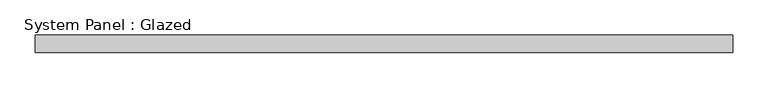
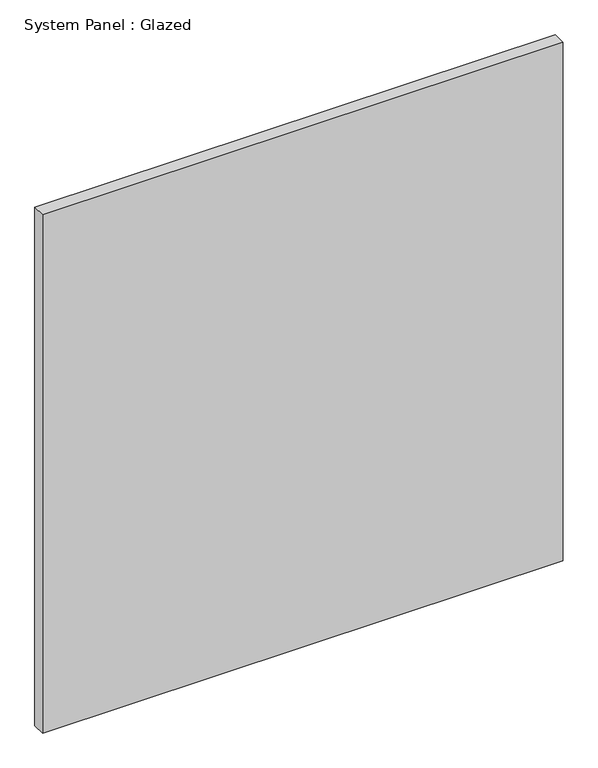
"""IFC4 building model written with IfcOpenShell, lengths in millimetres: plate geometry, System Panel : Glazed."""

from ifc_helpers import new_model, si_unit, origin, origin_with_axes, place, context, project, spatial, polyline, outline, extrude, source, transform, mapped, element, save


def system_panel_glazed_bdd68f76(model_context):
    return source(origin(), model_context, "Body", "SweptSolid", [
        extrude(outline(polyline([(494.887596, 24.5), (-494.887596, 24.5), (-494.887596, 49.5), (494.887596, 49.5), (494.887596, 24.5)])), origin_with_axes(), (0.0, 0.0, 1.0), 1041.4),
    ])


if __name__ == "__main__":
    model = new_model("IFC4")
    model_context = context("Model", 3, world=origin())
    ifc_project = project(units=[si_unit("LENGTHUNIT", "METRE", prefix="MILLI")], contexts=[model_context])
    site = spatial("IfcSite", under=ifc_project)
    building = spatial("IfcBuilding", under=site)
    placement = place(None, origin())
    system_panel_glazed_shape = system_panel_glazed_bdd68f76(model_context)
    element("IfcPlate", 1, ObjectType="System Panel : Glazed", at=placement, inside=building, context=model_context, shape_type="MappedRepresentation", body=[
        mapped(system_panel_glazed_shape, transform((0.0, 0.0, 0.0), x_axis=(1.0, 0.0, 0.0), y_axis=(0.0, 1.0, 0.0), z_axis=(0.0, 0.0, 1.0))),
    ])
    save(model, "model.ifc")

# Revit data of these elements
# Type "System Panel : Glazed"
#   Keynote = "H11"
#   Construction Type Id = "GSP4R"
#   Analytic Construction = "1/8 in Pilkington single glazing"
#   Visual Light Transmittance = 0.9
#   Solar Heat Gain Coefficient = 0.86
#   Heat Transfer Coefficient (U) = 6.7069 W/(m²·K)
#   Define Thermal Properties by = 1
# Element 1 (IfcPlate, "System Panel : Glazed")
#   Materials on its faces: "Glass"
# Materials
#   "Glass": class "Glass", colour RGB 0 128 192, transparency 0.9, Description = "Soda Lime Glass", Cost = 0
